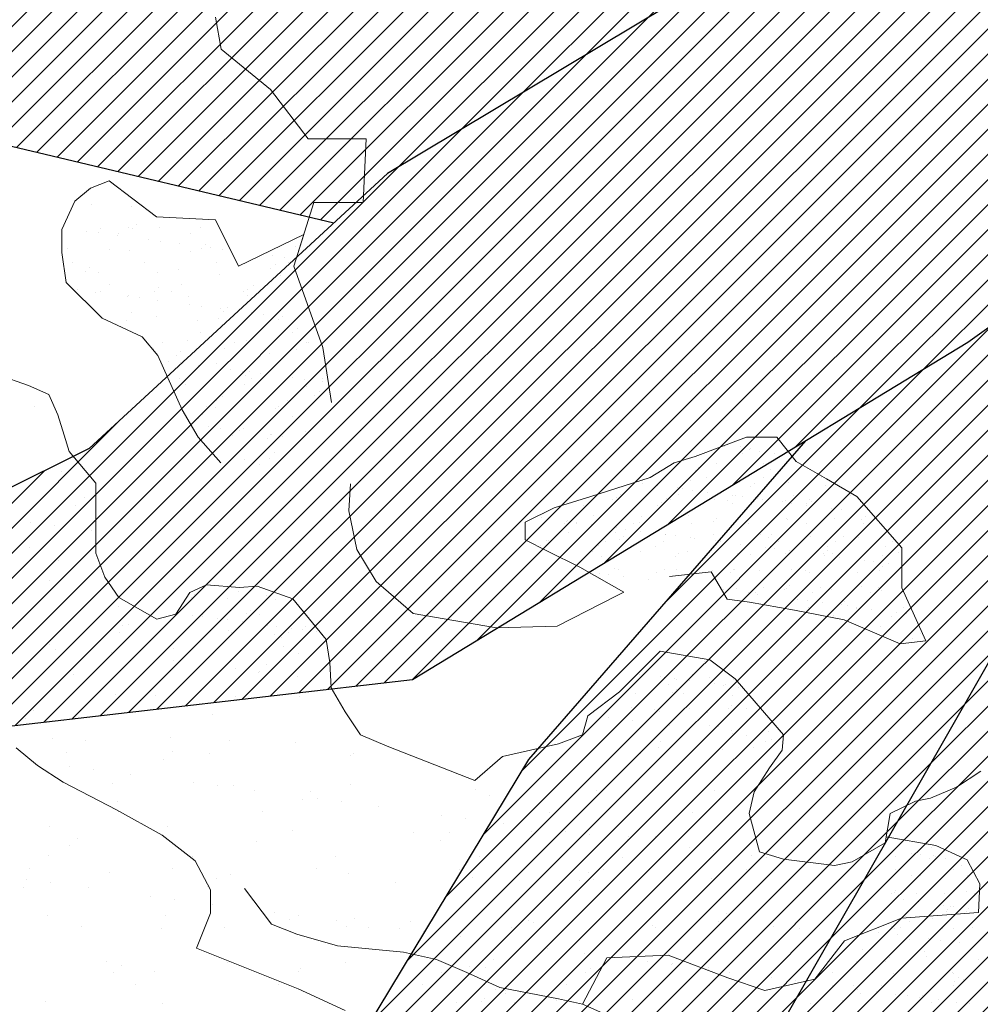
# Model space of a CAD drawing. Units: inches. Extents: x 1986 to 21484, y -1816 to 2016.
# Tile 15 of 85: x 2158.236 to 2166.564, y 1873.899 to 1882.437. Entities that reach past the tile are written whole.
import ezdxf

# ---------------------------------------------------------------- set-up
doc = ezdxf.new("R2010")
doc.units = ezdxf.units.IN
doc.layers.add('L-PLNT', color=84, linetype='Continuous', lineweight=13)
doc.layers.add('vfolhas', color=114, linetype='Continuous', lineweight=5)
for name, color, linetype in [('vfolha', 72, 'Continuous'), ('vfolha2', 110, 'Continuous'), ('vfolhas2', 102, 'Continuous')]:
    doc.layers.add(name, color=color, linetype=linetype)
pattern_1 = [(45, (-2446.5133113, 50.986076), (-0.004419417382, 0.004419417382), [])]

# ---------------------------------------------------------------- blocks, each defined once
blk = doc.blocks.new('arbusto_PB_verde_grande')
at = {"layer": 'vfolha2'}
h = blk.add_hatch(dxfattribs=at)
h.set_pattern_fill('ANSI31', color=256, scale=0.05, style=0)
h.set_pattern_definition(pattern_1)
h.paths.add_polyline_path([(0.02944, 0.35651), (0.00028, 0.09048), (0.02625, -0.03934), (0.047, 0.06233), (0.06189, 0.09731), (0.09372, 0.26573), (0.09955, 0.43473), (0.08789, 0.61313), (0.0645, 0.72266), (0.04988, 0.6851), (0.0236, 0.51294)])
h.paths.add_polyline_path([(0.30106, 0.43789), (0.14225, 0.24871), (0.26685, 0.30022)])
h.paths.add_polyline_path([(0.37995, 0.22817), (0.23697, 0.15193), (0.18428, 0.09364), (0.11122, 0.04358), (0.02625, -0.03934), (0.28061, 0.04667), (0.36829, 0.07798), (0.46756, 0.11239), (0.61068, 0.19376), (0.71585, 0.27823), (0.55813, 0.25948)])
h.paths.add_polyline_path([(0.56101, -0.29441), (0.72752, -0.32573), (0.59024, -0.2412), (0.42962, -0.15982), (0.02625, -0.03934), (0.14922, -0.14107), (0.18838, -0.16604), (0.41501, -0.24435)])
h.paths.add_polyline_path([(-0.27429, -0.44776), (-0.30352, -0.72628), (-0.23923, -0.64175), (-0.15457, -0.45716), (0.02625, -0.03934), (-0.16328, -0.25376)])
h.paths.add_polyline_path([(-0.51963, -0.24744), (-0.67736, -0.32573), (-0.59558, -0.35072), (-0.40574, -0.32882), (-0.21007, -0.20995), (0.02625, -0.03934), (-0.14874, -0.06595), (-0.31518, -0.09101), (-0.41452, -0.15048)])
h.paths.add_polyline_path([(-0.52546, 0.25007), (-0.70947, 0.24698), (-0.51963, 0.1093), (-0.32979, 0.02167), (-0.07567, -0.0128), (-0.04234, -0.02148), (-0.35024, 0.1312)])
at = {"layer": 'vfolhas'}
h = blk.add_hatch(dxfattribs=at)
h.set_pattern_fill('ANSI31', color=256, scale=0.05, style=0)
h.set_pattern_definition(pattern_1)
h.paths.add_polyline_path([(-0.57219, 0.06233), (-0.7153, 0.10298), (-0.67736, 0.08107), (-0.62769, 0.01536), (-0.56347, -0.04095), (-0.26461, -0.0834), (-0.14874, -0.06595), (-0.10151, -0.05877), (-0.20418, -0.0472), (-0.40279, -0.00339)])
h.paths.add_polyline_path([(-0.56347, -0.04095), (-0.58279, -0.02401), (-0.72992, -0.09726), (-0.4334, -0.1679), (-0.41452, -0.15048), (-0.31518, -0.09101), (-0.26461, -0.0834)])
h.paths.add_polyline_path([(-0.2769, -0.47267), (-0.27429, -0.44776), (-0.16328, -0.25376), (0.02625, -0.03934), (-0.21007, -0.20995), (-0.2672, -0.24466), (-0.36485, -0.35697), (-0.42907, -0.46341), (-0.47586, -0.60425), (-0.37946, -0.57603)])
at = {"layer": 'vfolha'}
blk.add_line((-0.2672, -0.24466), (-0.36485, -0.35697), dxfattribs=at)
at = {"layer": 'vfolha2'}
for p, q in [((-0.21007, -0.20995), (0.02625, -0.03934)), ((-0.31518, -0.09101), (-0.41452, -0.15048)), ((-0.41452, -0.15048), (-0.51963, -0.24744)), ((-0.40574, -0.32882), (-0.21007, -0.20995)), ((-0.51963, -0.24744), (-0.67736, -0.32573)), ((-0.16328, -0.25376), (-0.27429, -0.44776)), ((-0.59558, -0.35072), (-0.40574, -0.32882))]:
    blk.add_line(p, q, dxfattribs=at)
at = {"layer": 'vfolhas2'}
for p, q in [((-0.72992, -0.09726), (-0.4334, -0.1679)), ((-0.36485, -0.35697), (-0.42907, -0.46341))]:
    blk.add_line(p, q, dxfattribs=at)
blk = doc.blocks.new('PLANT-SHRUB')
for p, q in [((2159.933, 1882.4585), (2159.9833, 1882.1822)), ((2159.9833, 1882.1822), (2160.4105, 1881.8306)), ((2159.9833, 1882.1822), (2159.9833, 1882.1822)), ((2160.4105, 1881.8306), (2160.7373, 1881.4037)), ((2160.4105, 1881.8306), (2160.4105, 1881.8306)), ((2160.7373, 1881.4037), (2161.24, 1881.4037)), ((2161.24, 1881.4037), (2161.2149, 1880.8511)), ((2159.0126, 1881.0382), (2158.8512, 1880.9762)), ((2159.4223, 1880.7281), (2159.0126, 1881.0382)), ((2158.8512, 1880.9762), (2158.7146, 1880.8646)), ((2158.7146, 1880.8646), (2158.6029, 1880.6164)), ((2160.7876, 1880.8511), (2160.6116, 1880.2986)), ((2161.2149, 1880.8511), (2160.7876, 1880.8511)), ((2158.8595, 1880.8325), (2158.8595, 1880.8325)), ((2159.2032, 1880.8173), (2159.2032, 1880.8173)), ((2159.933, 1880.7004), (2159.4223, 1880.7281)), ((2159.933, 1880.7004), (2159.933, 1880.7004)), ((2160.1341, 1880.2986), (2159.933, 1880.7004)), ((2158.6029, 1880.6164), (2158.6029, 1880.4179)), ((2158.8149, 1880.6018), (2158.8149, 1880.6018)), ((2158.9189, 1880.5881), (2158.9189, 1880.5881)), ((2158.9329, 1880.6299), (2158.9329, 1880.6299)), ((2159.0941, 1880.5844), (2159.0941, 1880.5844)), ((2159.1784, 1880.6381), (2159.1784, 1880.6381)), ((2159.2123, 1880.6297), (2159.2123, 1880.6297)), ((2159.2491, 1880.6634), (2159.2491, 1880.6634)), ((2159.4441, 1880.6323), (2159.4441, 1880.6323)), ((2159.7165, 1880.5832), (2159.7165, 1880.5832)), ((2159.8007, 1880.6369), (2159.8007, 1880.6369)), ((2159.0813, 1880.5667), (2159.0813, 1880.5667)), ((2159.3528, 1880.5309), (2159.3528, 1880.5309)), ((2159.4568, 1880.5173), (2159.4568, 1880.5173)), ((2160.6996, 1880.5749), (2160.1341, 1880.2986)), ((2160.6116, 1880.2986), (2160.6996, 1880.5749)), ((2160.6996, 1880.5749), (2160.6996, 1880.5749)), ((2158.6029, 1880.4179), (2158.6401, 1880.1574)), ((2158.6508, 1880.4516), (2158.6508, 1880.4516)), ((2159.0134, 1880.4474), (2159.0134, 1880.4474)), ((2159.1906, 1880.4322), (2159.1906, 1880.4322)), ((2159.6193, 1880.4959), (2159.6193, 1880.4959)), ((2159.7137, 1880.4255), (2159.7137, 1880.4255)), ((2159.813, 1880.4543), (2159.813, 1880.4543)), ((2159.8498, 1880.488), (2159.8498, 1880.488)), ((2159.8907, 1880.4601), (2159.8907, 1880.4601)), ((2159.9947, 1880.4464), (2159.9947, 1880.4464)), ((2160.6244, 1880.472), (2160.6244, 1880.472)), ((2158.6981, 1880.3321), (2158.6981, 1880.3321)), ((2159.3204, 1880.3309), (2159.3204, 1880.3309)), ((2159.9427, 1880.3298), (2159.9427, 1880.3298)), ((2160.4286, 1880.3893), (2160.4286, 1880.3893)), ((2160.5326, 1880.3756), (2160.5326, 1880.3756)), ((2160.565, 1880.3287), (2160.565, 1880.3287)), ((2158.8027, 1880.2544), (2158.8027, 1880.2544)), ((2158.8395, 1880.2881), (2158.8395, 1880.2881)), ((2158.9203, 1880.2448), (2158.9203, 1880.2448)), ((2159.4315, 1880.2473), (2159.4315, 1880.2473)), ((2159.6141, 1880.272), (2159.6141, 1880.272)), ((2160.1341, 1880.2986), (2160.1341, 1880.2986)), ((2160.4137, 1880.2789), (2160.4137, 1880.2789)), ((2160.4506, 1880.3126), (2160.4506, 1880.3126)), ((2160.6116, 1880.2986), (2160.863, 1879.5954)), ((2160.6116, 1880.2986), (2160.6116, 1880.2986)), ((2158.6401, 1880.1574), (2158.9505, 1879.8472)), ((2159.9713, 1880.2278), (2159.9713, 1880.2278)), ((2160.4944, 1880.2212), (2160.4944, 1880.2212)), ((2158.7346, 1880.0949), (2158.7346, 1880.0949)), ((2158.8971, 1880.0735), (2158.8971, 1880.0735)), ((2158.9328, 1880.084), (2158.9328, 1880.084)), ((2159.017, 1880.1377), (2159.017, 1880.1377)), ((2159.4034, 1880.079), (2159.4034, 1880.079)), ((2159.4402, 1880.1127), (2159.4402, 1880.1127)), ((2159.5551, 1880.0828), (2159.5551, 1880.0828)), ((2159.6393, 1880.1365), (2159.6393, 1880.1365)), ((2160.1774, 1880.0817), (2160.1774, 1880.0817)), ((2160.2148, 1880.0966), (2160.2148, 1880.0966)), ((2160.2617, 1880.1354), (2160.2617, 1880.1354)), ((2159.1685, 1880.0378), (2159.1685, 1880.0378)), ((2159.178, 1880.0472), (2159.178, 1880.0472)), ((2159.2725, 1880.0241), (2159.2725, 1880.0241)), ((2159.435, 1880.0027), (2159.435, 1880.0027)), ((2159.7011, 1880.0405), (2159.7011, 1880.0405)), ((2160.2123, 1880.0429), (2160.2123, 1880.0429)), ((2159.7064, 1879.967), (2159.7064, 1879.967)), ((2159.8105, 1879.9533), (2159.8105, 1879.9533)), ((2159.9729, 1879.9319), (2159.9729, 1879.9319)), ((2160.0041, 1879.9036), (2160.0041, 1879.9036)), ((2160.041, 1879.9373), (2160.041, 1879.9373)), ((2158.9505, 1879.8472), (2159.2982, 1879.686)), ((2159.159, 1879.8305), (2159.159, 1879.8305)), ((2159.2045, 1879.8967), (2159.2045, 1879.8967)), ((2159.419, 1879.8622), (2159.419, 1879.8622)), ((2159.7813, 1879.8294), (2159.7813, 1879.8294)), ((2159.9587, 1879.8428), (2159.9587, 1879.8428)), ((2160.2444, 1879.8962), (2160.2444, 1879.8962)), ((2160.3484, 1879.8825), (2160.3484, 1879.8825)), ((2160.4036, 1879.8283), (2160.4036, 1879.8283)), ((2160.4818, 1879.8361), (2160.4818, 1879.8361)), ((2160.5108, 1879.8611), (2160.5108, 1879.8611)), ((2160.6417, 1879.7619), (2160.6417, 1879.7619)), ((2159.2982, 1879.686), (2159.4348, 1879.5247)), ((2159.6885, 1879.6554), (2159.6885, 1879.6554)), ((2159.8052, 1879.7213), (2159.8052, 1879.7213)), ((2160.1997, 1879.6579), (2160.1997, 1879.6579)), ((2160.6049, 1879.7282), (2160.6049, 1879.7282)), ((2159.3937, 1879.5824), (2159.3937, 1879.5824)), ((2159.4779, 1879.6361), (2159.4779, 1879.6361)), ((2159.6314, 1879.562), (2159.6314, 1879.562)), ((2160.016, 1879.5813), (2160.016, 1879.5813)), ((2160.1003, 1879.635), (2160.1003, 1879.635)), ((2160.6383, 1879.5802), (2160.6383, 1879.5802)), ((2160.7226, 1879.6339), (2160.7226, 1879.6339)), ((2160.7394, 1879.6384), (2160.7394, 1879.6384)), ((2160.863, 1879.5954), (2160.9384, 1879.1182)), ((2159.4348, 1879.5247), (2159.6458, 1879.0532)), ((2159.4348, 1879.5247), (2159.4348, 1879.5247)), ((2159.5222, 1879.4738), (2159.5222, 1879.4738)), ((2159.5945, 1879.5283), (2159.5945, 1879.5283)), ((2160.406, 1879.5459), (2160.406, 1879.5459)), ((2159.6262, 1879.4601), (2159.6262, 1879.4601)), ((2159.7887, 1879.4388), (2159.7887, 1879.4388)), ((2159.9461, 1879.4578), (2159.9461, 1879.4578)), ((2160.0601, 1879.403), (2160.0601, 1879.403)), ((2160.1641, 1879.3893), (2160.1641, 1879.3893)), ((2160.4692, 1879.4511), (2160.4692, 1879.4511)), ((2158.0049, 1879.3737), (2158.3132, 1879.2637)), ((2159.6199, 1879.329), (2159.6199, 1879.329)), ((2160.1953, 1879.3529), (2160.1953, 1879.3529)), ((2160.2321, 1879.3866), (2160.2321, 1879.3866)), ((2160.2422, 1879.3278), (2160.2422, 1879.3278)), ((2160.3266, 1879.3679), (2160.3266, 1879.3679)), ((2160.598, 1879.3322), (2160.598, 1879.3322)), ((2160.702, 1879.3185), (2160.702, 1879.3185)), ((2160.8646, 1879.3267), (2160.8646, 1879.3267)), ((2158.3132, 1879.2637), (2158.4894, 1879.1867)), ((2159.6759, 1879.2704), (2159.6759, 1879.2704)), ((2160.1871, 1879.2728), (2160.1871, 1879.2728)), ((2160.7268, 1879.2534), (2160.7268, 1879.2534)), ((2160.8645, 1879.2971), (2160.8645, 1879.2971)), ((2158.4894, 1879.1867), (2158.5664, 1879.0106)), ((2159.9389, 1879.1346), (2159.9389, 1879.1346)), ((2159.9964, 1879.1706), (2159.9964, 1879.1706)), ((2160.5612, 1879.1334), (2160.5612, 1879.1334)), ((2160.796, 1879.1775), (2160.796, 1879.1775)), ((2160.8328, 1879.2112), (2160.8328, 1879.2112)), ((2158.3642, 1879.0832), (2158.3642, 1879.0832)), ((2159.6458, 1879.0532), (2159.7824, 1878.8175)), ((2159.8546, 1879.0809), (2159.8546, 1879.0809)), ((2159.9335, 1879.0727), (2159.9335, 1879.0727)), ((2160.4566, 1879.066), (2160.4566, 1879.066)), ((2160.4769, 1879.0798), (2160.4769, 1879.0798)), ((2158.5664, 1879.0106), (2158.6215, 1878.8346)), ((2159.7857, 1878.9775), (2159.7857, 1878.9775)), ((2159.8225, 1879.0113), (2159.8225, 1879.0113)), ((2160.5971, 1878.9952), (2160.5971, 1878.9952)), ((2159.8759, 1878.9099), (2159.8759, 1878.9099)), ((2159.9799, 1878.8962), (2159.9799, 1878.8962)), ((2160.1745, 1878.8878), (2160.1745, 1878.8878)), ((2158.6215, 1878.8346), (2158.6655, 1878.6916)), ((2159.7824, 1878.8175), (2159.9811, 1878.5942)), ((2160.0809, 1878.8274), (2160.0809, 1878.8274)), ((2160.1423, 1878.8748), (2160.1423, 1878.8748)), ((2160.3864, 1878.8022), (2160.3864, 1878.8022)), ((2160.4138, 1878.8391), (2160.4138, 1878.8391)), ((2160.4233, 1878.8359), (2160.4233, 1878.8359)), ((2160.5178, 1878.8254), (2160.5178, 1878.8254)), ((2160.6803, 1878.804), (2160.6803, 1878.804)), ((2160.7032, 1878.8263), (2160.7032, 1878.8263)), ((2160.7142, 1878.8683), (2160.7142, 1878.8683)), ((2164.0917, 1878.6487), (2164.5363, 1878.8153)), ((2164.5363, 1878.8153), (2164.8003, 1878.8153)), ((2164.8003, 1878.8153), (2164.967, 1878.607)), ((2164.8003, 1878.8153), (2164.8003, 1878.8153)), ((2164.3454, 1878.7354), (2164.3454, 1878.7354)), ((2164.4894, 1878.7345), (2164.4894, 1878.7345)), ((2164.5625, 1878.7068), (2164.5625, 1878.7068)), ((2164.5717, 1878.7149), (2164.5717, 1878.7149)), ((2158.6655, 1878.6916), (2158.8968, 1878.4165)), ((2159.9209, 1878.6877), (2159.9209, 1878.6877)), ((2160.1875, 1878.6199), (2160.1875, 1878.6199)), ((2160.3998, 1878.633), (2160.3998, 1878.633)), ((2160.444, 1878.681), (2160.444, 1878.681)), ((2163.9111, 1878.5931), (2164.0917, 1878.6487)), ((2164.2631, 1878.6802), (2164.2631, 1878.6802)), ((2164.5043, 1878.672), (2164.5043, 1878.672)), ((2164.6457, 1878.6958), (2164.6457, 1878.6958)), ((2164.7757, 1878.6787), (2164.7757, 1878.6787)), ((2164.9028, 1878.6857), (2164.9028, 1878.6857)), ((2159.9811, 1878.5942), (2159.9811, 1878.5942)), ((2160.3155, 1878.5794), (2160.3155, 1878.5794)), ((2163.7026, 1878.4682), (2163.9111, 1878.5931)), ((2164.124, 1878.5527), (2164.124, 1878.5527)), ((2164.2732, 1878.5846), (2164.2732, 1878.5846)), ((2164.6821, 1878.5866), (2164.6821, 1878.5866)), ((2164.7437, 1878.5398), (2164.7437, 1878.5398)), ((2164.967, 1878.607), (2165.231, 1878.4543)), ((2158.5998, 1878.5173), (2158.5998, 1878.5173)), ((2163.1885, 1878.3016), (2163.7026, 1878.4682)), ((2163.7026, 1878.4682), (2163.7026, 1878.4682)), ((2164.0946, 1878.5257), (2164.0946, 1878.5257)), ((2164.1874, 1878.4701), (2164.1874, 1878.4701)), ((2164.6853, 1878.4692), (2164.6853, 1878.4692)), ((2165.1831, 1878.4683), (2165.1831, 1878.4683)), ((2165.231, 1878.4543), (2165.495, 1878.3016)), ((2158.8968, 1878.4165), (2158.8968, 1878.0974)), ((2161.1044, 1878.4126), (2161.0905, 1878.1766)), ((2163.6377, 1878.4146), (2163.6377, 1878.4146)), ((2163.6385, 1878.4401), (2163.6385, 1878.4401)), ((2163.7676, 1878.3975), (2163.7676, 1878.3975)), ((2163.9355, 1878.3799), (2163.9355, 1878.3799)), ((2163.9848, 1878.3689), (2163.9848, 1878.3689)), ((2164.0475, 1878.4421), (2164.0475, 1878.4421)), ((2164.4793, 1878.4265), (2164.4793, 1878.4265)), ((2164.5752, 1878.3854), (2164.5752, 1878.3854)), ((2164.6046, 1878.4124), (2164.6046, 1878.4124)), ((2164.8978, 1878.4212), (2164.8978, 1878.4212)), ((2165.2243, 1878.3995), (2165.2243, 1878.3995)), ((2158.7944, 1878.2944), (2158.7944, 1878.2944)), ((2162.869, 1878.2044), (2163.1885, 1878.3016)), ((2163.1885, 1878.3016), (2163.1885, 1878.3016)), ((2163.4129, 1878.2975), (2163.4129, 1878.2975)), ((2163.4468, 1878.3164), (2163.4468, 1878.3164)), ((2163.8446, 1878.2819), (2163.8446, 1878.2819)), ((2163.9447, 1878.3155), (2163.9447, 1878.3155)), ((2164.068, 1878.358), (2164.068, 1878.358)), ((2164.198, 1878.3409), (2164.198, 1878.3409)), ((2164.4151, 1878.3123), (2164.4151, 1878.3123)), ((2164.4426, 1878.3146), (2164.4426, 1878.3146)), ((2164.4983, 1878.3013), (2164.4983, 1878.3013)), ((2164.6283, 1878.2842), (2164.6283, 1878.2842)), ((2164.6721, 1878.2786), (2164.6721, 1878.2786)), ((2164.9404, 1878.3137), (2164.9404, 1878.3137)), ((2165.4383, 1878.3128), (2165.4383, 1878.3128)), ((2165.495, 1878.3016), (2165.8841, 1877.8573)), ((2158.7207, 1878.2269), (2158.7207, 1878.2269)), ((2162.6189, 1878.0794), (2162.869, 1878.2044)), ((2163.1272, 1878.22), (2163.1272, 1878.22)), ((2163.1272, 1878.22), (2163.1272, 1878.22)), ((2163.3794, 1878.2735), (2163.3794, 1878.2735)), ((2163.7669, 1878.2255), (2163.7669, 1878.2255)), ((2163.7964, 1878.2525), (2163.7964, 1878.2525)), ((2163.8773, 1878.2725), (2163.8773, 1878.2725)), ((2164.2631, 1878.2766), (2164.2631, 1878.2766)), ((2164.3751, 1878.2716), (2164.3751, 1878.2716)), ((2164.416, 1878.2396), (2164.416, 1878.2396)), ((2164.8455, 1878.2556), (2164.8455, 1878.2556)), ((2164.873, 1878.2707), (2164.873, 1878.2707)), ((2164.9287, 1878.2447), (2164.9287, 1878.2447)), ((2165.0558, 1878.2451), (2165.0558, 1878.2451)), ((2165.0586, 1878.2275), (2165.0586, 1878.2275)), ((2165.0852, 1878.2721), (2165.0852, 1878.2721)), ((2165.1039, 1878.263), (2165.1039, 1878.263)), ((2165.2758, 1878.199), (2165.2758, 1878.199)), ((2165.3708, 1878.2698), (2165.3708, 1878.2698)), ((2165.5223, 1878.2577), (2165.5223, 1878.2577)), ((2161.0905, 1878.1766), (2161.1599, 1877.8434)), ((2162.7596, 1878.1163), (2162.7596, 1878.1163)), ((2162.7782, 1878.153), (2162.7782, 1878.153)), ((2163.21, 1878.1374), (2163.21, 1878.1374)), ((2163.6285, 1878.1321), (2163.6285, 1878.1321)), ((2164.0374, 1878.134), (2164.0374, 1878.134)), ((2164.277, 1878.1121), (2164.277, 1878.1121)), ((2164.4692, 1878.1185), (2164.4692, 1878.1185)), ((2164.8877, 1878.1131), (2164.8877, 1878.1131)), ((2165.2966, 1878.1151), (2165.2966, 1878.1151)), ((2165.359, 1878.188), (2165.359, 1878.188)), ((2165.489, 1878.1709), (2165.489, 1878.1709)), ((2165.5658, 1878.1318), (2165.5658, 1878.1318)), ((2158.3275, 1878.0789), (2158.3275, 1878.0789)), ((2158.5356, 1878.0515), (2158.5356, 1878.0515)), ((2158.8968, 1878.0974), (2158.8968, 1877.8113)), ((2162.6189, 1877.9267), (2162.6189, 1878.0794)), ((2162.9587, 1878.0655), (2162.9587, 1878.0655)), ((2162.9587, 1878.0655), (2162.9587, 1878.0655)), ((2162.9767, 1878.0877), (2162.9767, 1878.0877)), ((2162.9767, 1878.0877), (2162.9767, 1878.0877)), ((2162.9881, 1878.0925), (2162.9881, 1878.0925)), ((2162.9881, 1878.0925), (2162.9881, 1878.0925)), ((2163.0599, 1878.0768), (2163.0599, 1878.0768)), ((2163.0599, 1878.0768), (2163.0599, 1878.0768)), ((2163.0626, 1878.0716), (2163.0626, 1878.0716)), ((2163.0626, 1878.0716), (2163.0626, 1878.0716)), ((2163.1899, 1878.0596), (2163.1899, 1878.0596)), ((2163.4071, 1878.0311), (2163.4071, 1878.0311)), ((2163.5604, 1878.0707), (2163.5604, 1878.0707)), ((2163.6078, 1878.0796), (2163.6078, 1878.0796)), ((2164.0583, 1878.0698), (2164.0583, 1878.0698)), ((2164.2475, 1878.0851), (2164.2475, 1878.0851)), ((2164.5561, 1878.0689), (2164.5561, 1878.0689)), ((2164.8966, 1878.0993), (2164.8966, 1878.0993)), ((2165.054, 1878.068), (2165.054, 1878.068)), ((2165.5363, 1878.1048), (2165.5363, 1878.1048)), ((2165.5518, 1878.0671), (2165.5518, 1878.0671)), ((2158.8605, 1878.0087), (2158.8605, 1878.0087)), ((2162.9938, 1877.9875), (2162.9938, 1877.9875)), ((2162.9938, 1877.9875), (2162.9938, 1877.9875)), ((2163.4028, 1877.9895), (2163.4028, 1877.9895)), ((2163.4687, 1877.9522), (2163.4687, 1877.9522)), ((2163.4903, 1878.0201), (2163.4903, 1878.0201)), ((2163.6202, 1878.003), (2163.6202, 1878.003)), ((2163.8346, 1877.9739), (2163.8346, 1877.9739)), ((2163.8374, 1877.9744), (2163.8374, 1877.9744)), ((2163.9206, 1877.9634), (2163.9206, 1877.9634)), ((2164.0506, 1877.9463), (2164.0506, 1877.9463)), ((2164.0884, 1877.9393), (2164.0884, 1877.9393)), ((2164.253, 1877.9686), (2164.253, 1877.9686)), ((2164.662, 1877.9705), (2164.662, 1877.9705)), ((2164.7281, 1877.9448), (2164.7281, 1877.9448)), ((2164.7575, 1877.9718), (2164.7575, 1877.9718)), ((2165.0938, 1877.955), (2165.0938, 1877.955)), ((2165.3772, 1877.959), (2165.3772, 1877.959)), ((2165.5123, 1877.9496), (2165.5123, 1877.9496)), ((2158.3229, 1877.8624), (2158.3229, 1877.8624)), ((2162.8134, 1877.8295), (2162.6189, 1877.9267)), ((2162.7525, 1877.874), (2162.7525, 1877.874)), ((2162.7525, 1877.874), (2162.7525, 1877.874)), ((2162.7995, 1877.9197), (2162.7995, 1877.9197)), ((2162.7995, 1877.9197), (2162.7995, 1877.9197)), ((2162.8199, 1877.917), (2162.8199, 1877.917)), ((2162.8199, 1877.917), (2162.8199, 1877.917)), ((2163.2503, 1877.8731), (2163.2503, 1877.8731)), ((2163.3177, 1877.9161), (2163.3177, 1877.9161)), ((2163.4392, 1877.9252), (2163.4392, 1877.9252)), ((2163.7482, 1877.8722), (2163.7482, 1877.8722)), ((2163.8156, 1877.9152), (2163.8156, 1877.9152)), ((2164.246, 1877.8713), (2164.246, 1877.8713)), ((2164.2677, 1877.9177), (2164.2677, 1877.9177)), ((2164.3134, 1877.9143), (2164.3134, 1877.9143)), ((2164.3509, 1877.9068), (2164.3509, 1877.9068)), ((2164.4809, 1877.8897), (2164.4809, 1877.8897)), ((2164.6981, 1877.8611), (2164.6981, 1877.8611)), ((2164.7439, 1877.8704), (2164.7439, 1877.8704)), ((2164.8113, 1877.9134), (2164.8113, 1877.9134)), ((2165.2417, 1877.8695), (2165.2417, 1877.8695)), ((2165.3091, 1877.9125), (2165.3091, 1877.9125)), ((2165.7396, 1877.8686), (2165.7396, 1877.8686)), ((2165.807, 1877.9116), (2165.807, 1877.9116)), ((2165.8841, 1877.8573), (2165.8841, 1877.5102)), ((2158.8968, 1877.8113), (2158.9739, 1877.6023)), ((2161.1599, 1877.8434), (2161.3267, 1877.5657)), ((2163.0913, 1877.6907), (2162.8134, 1877.8295)), ((2163.1999, 1877.8294), (2163.1999, 1877.8294)), ((2163.2801, 1877.7794), (2163.2801, 1877.7794)), ((2163.6184, 1877.824), (2163.6184, 1877.824)), ((2163.9198, 1877.7849), (2163.9198, 1877.7849)), ((2163.9493, 1877.8119), (2163.9493, 1877.8119)), ((2164.0274, 1877.826), (2164.0274, 1877.826)), ((2164.4591, 1877.8104), (2164.4591, 1877.8104)), ((2164.569, 1877.799), (2164.569, 1877.799)), ((2164.7813, 1877.8501), (2164.7813, 1877.8501)), ((2164.8776, 1877.8051), (2164.8776, 1877.8051)), ((2164.9112, 1877.833), (2164.9112, 1877.833)), ((2165.1284, 1877.8044), (2165.1284, 1877.8044)), ((2165.2087, 1877.8045), (2165.2087, 1877.8045)), ((2165.2116, 1877.7935), (2165.2116, 1877.7935)), ((2165.2381, 1877.8315), (2165.2381, 1877.8315)), ((2165.2866, 1877.807), (2165.2866, 1877.807)), ((2165.3416, 1877.7764), (2165.3416, 1877.7764)), ((2165.7184, 1877.7915), (2165.7184, 1877.7915)), ((2165.8578, 1877.8187), (2165.8578, 1877.8187)), ((2158.5746, 1877.7472), (2158.5746, 1877.7472)), ((2163.4729, 1877.4726), (2163.0913, 1877.6907)), ((2163.3927, 1877.6814), (2163.3927, 1877.6814)), ((2165.5587, 1877.7478), (2165.5587, 1877.7478)), ((2165.6419, 1877.7368), (2165.6419, 1877.7368)), ((2165.7187, 1877.6912), (2165.7187, 1877.6912)), ((2165.7719, 1877.7197), (2165.7719, 1877.7197)), ((2158.9739, 1877.6023), (2159.095, 1877.4262)), ((2163.2597, 1877.6365), (2163.2597, 1877.6365)), ((2163.3429, 1877.6256), (2163.3429, 1877.6256)), ((2163.4313, 1877.6704), (2163.4313, 1877.6704)), ((2163.4729, 1877.6085), (2163.4729, 1877.6085)), ((2163.7607, 1877.6391), (2163.7607, 1877.6391)), ((2163.8245, 1877.6659), (2163.8245, 1877.6659)), ((2164.2306, 1877.649), (2163.8694, 1877.6074)), ((2163.9292, 1877.6695), (2163.9292, 1877.6695)), ((2164.3696, 1877.413), (2164.2306, 1877.649)), ((2164.243, 1877.6605), (2164.243, 1877.6605)), ((2164.4004, 1877.6446), (2164.4004, 1877.6446)), ((2164.427, 1877.6686), (2164.427, 1877.6686)), ((2164.4299, 1877.6716), (2164.4299, 1877.6716)), ((2164.6519, 1877.6625), (2164.6519, 1877.6625)), ((2164.9249, 1877.6676), (2164.9249, 1877.6676)), ((2165.0495, 1877.6587), (2165.0495, 1877.6587)), ((2165.0837, 1877.6469), (2165.0837, 1877.6469)), ((2165.4227, 1877.6667), (2165.4227, 1877.6667)), ((2165.5022, 1877.6416), (2165.5022, 1877.6416)), ((2165.6892, 1877.6642), (2165.6892, 1877.6642)), ((2158.4939, 1877.5754), (2158.4939, 1877.5754)), ((2159.7116, 1877.4703), (2159.8548, 1877.5363)), ((2159.8548, 1877.5363), (2160.1411, 1877.5143)), ((2160.1411, 1877.5143), (2160.2952, 1877.5253)), ((2160.1411, 1877.5143), (2160.1411, 1877.5143)), ((2160.2952, 1877.5253), (2160.6035, 1877.4152)), ((2161.3267, 1877.5657), (2161.6462, 1877.2881)), ((2163.69, 1877.5799), (2163.69, 1877.5799)), ((2164.6822, 1877.513), (2164.6822, 1877.513)), ((2164.9105, 1877.5313), (2164.9105, 1877.5313)), ((2165.18, 1877.5121), (2165.18, 1877.5121)), ((2165.5301, 1877.5184), (2165.5301, 1877.5184)), ((2165.6779, 1877.5112), (2165.6779, 1877.5112)), ((2165.8841, 1877.5102), (2166.0925, 1877.052)), ((2159.095, 1877.4262), (2159.4253, 1877.2392)), ((2159.5905, 1877.2832), (2159.7116, 1877.4703)), ((2159.7256, 1877.4257), (2159.7256, 1877.4257)), ((2159.7551, 1877.4527), (2159.7551, 1877.4527)), ((2160.1341, 1877.4782), (2160.1341, 1877.4782)), ((2160.3748, 1877.4399), (2160.3748, 1877.4399)), ((2162.8967, 1877.177), (2163.4108, 1877.4408)), ((2163.4108, 1877.4408), (2163.4729, 1877.4726)), ((2163.4108, 1877.4408), (2163.4108, 1877.4408)), ((2164.3335, 1877.4952), (2164.3335, 1877.4952)), ((2164.4491, 1877.5024), (2164.4491, 1877.5024)), ((2164.5507, 1877.4666), (2164.5507, 1877.4666)), ((2164.6148, 1877.4701), (2164.6148, 1877.4701)), ((2164.6339, 1877.4556), (2164.6339, 1877.4556)), ((2164.7638, 1877.4385), (2164.7638, 1877.4385)), ((2164.8675, 1877.497), (2164.8675, 1877.497)), ((2164.881, 1877.5043), (2164.881, 1877.5043)), ((2165.1126, 1877.4692), (2165.1126, 1877.4692)), ((2165.2765, 1877.499), (2165.2765, 1877.499)), ((2165.6105, 1877.4683), (2165.6105, 1877.4683)), ((2165.7083, 1877.4835), (2165.7083, 1877.4835)), ((2159.0899, 1877.3518), (2159.0899, 1877.3518)), ((2160.0368, 1877.4146), (2160.0368, 1877.4146)), ((2160.4553, 1877.4093), (2160.4553, 1877.4093)), ((2160.6035, 1877.4152), (2160.8925, 1877.0609)), ((2164.5641, 1877.3852), (2164.3696, 1877.413)), ((2164.5641, 1877.3852), (2164.5641, 1877.3852)), ((2164.9531, 1877.3158), (2164.5641, 1877.3852)), ((2164.7219, 1877.3585), (2164.7219, 1877.3585)), ((2164.981, 1877.4099), (2164.981, 1877.4099)), ((2165.0642, 1877.399), (2165.0642, 1877.399)), ((2165.0736, 1877.3389), (2165.0736, 1877.3389)), ((2165.1942, 1877.3819), (2165.1942, 1877.3819)), ((2165.3616, 1877.3639), (2165.3616, 1877.3639)), ((2165.391, 1877.391), (2165.391, 1877.391)), ((2165.4113, 1877.3533), (2165.4113, 1877.3533)), ((2165.4945, 1877.3423), (2165.4945, 1877.3423)), ((2159.4253, 1877.2392), (2159.5905, 1877.2832)), ((2159.6054, 1877.2898), (2159.6054, 1877.2898)), ((2159.7354, 1877.2727), (2159.7354, 1877.2727)), ((2159.8172, 1877.2764), (2159.8172, 1877.2764)), ((2159.8206, 1877.2647), (2159.8206, 1877.2647)), ((2160.2062, 1877.2854), (2160.2062, 1877.2854)), ((2160.2296, 1877.2667), (2160.2296, 1877.2667)), ((2160.2357, 1877.3124), (2160.2357, 1877.3124)), ((2160.3151, 1877.2755), (2160.3151, 1877.2755)), ((2161.6462, 1877.2881), (2162.3688, 1877.1631)), ((2165.3839, 1877.2325), (2164.9531, 1877.3158)), ((2165.2936, 1877.2664), (2165.2936, 1877.2664)), ((2165.4921, 1877.3336), (2165.4921, 1877.3336)), ((2165.6245, 1877.3252), (2165.6245, 1877.3252)), ((2165.7915, 1877.2655), (2165.7915, 1877.2655)), ((2165.8416, 1877.2966), (2165.8416, 1877.2966)), ((2165.9011, 1877.3355), (2165.9011, 1877.3355)), ((2165.9249, 1877.2857), (2165.9249, 1877.2857)), ((2159.1318, 1877.1866), (2159.1318, 1877.1866)), ((2159.1767, 1877.193), (2159.1767, 1877.193)), ((2159.4253, 1877.2392), (2159.4253, 1877.2392)), ((2159.9526, 1877.2441), (2159.9526, 1877.2441)), ((2160.0358, 1877.2331), (2160.0358, 1877.2331)), ((2160.1657, 1877.216), (2160.1657, 1877.216)), ((2160.3829, 1877.1874), (2160.3829, 1877.1874)), ((2160.4661, 1877.1765), (2160.4661, 1877.1765)), ((2160.6614, 1877.2511), (2160.6614, 1877.2511)), ((2160.7163, 1877.1721), (2160.7163, 1877.1721)), ((2162.3688, 1877.1631), (2162.8967, 1877.177)), ((2165.8702, 1877.0243), (2165.3839, 1877.2325)), ((2165.6982, 1877.1754), (2165.6982, 1877.1754)), ((2165.8422, 1877.2236), (2165.8422, 1877.2236)), ((2165.8716, 1877.2506), (2165.8716, 1877.2506)), ((2159.103, 1877.1255), (2159.103, 1877.1255)), ((2160.0471, 1877.1396), (2160.0471, 1877.1396)), ((2160.0724, 1877.1208), (2160.0724, 1877.1208)), ((2160.4452, 1877.1013), (2160.4452, 1877.1013)), ((2160.5702, 1877.1199), (2160.5702, 1877.1199)), ((2160.5961, 1877.1594), (2160.5961, 1877.1594)), ((2160.6868, 1877.1451), (2160.6868, 1877.1451)), ((2160.8132, 1877.1308), (2160.8132, 1877.1308)), ((2160.8541, 1877.1032), (2160.8541, 1877.1032)), ((2166.0466, 1877.11), (2166.0466, 1877.11)), ((2158.492, 1877.0224), (2158.492, 1877.0224)), ((2158.9632, 1877.0793), (2158.9632, 1877.0793)), ((2160.5028, 1877.077), (2160.5028, 1877.077)), ((2160.5277, 1876.9993), (2160.5277, 1876.9993)), ((2160.8925, 1877.0609), (2160.9255, 1876.8629)), ((2166.0925, 1877.052), (2165.8702, 1877.0243)), ((2165.891, 1877.0275), (2165.891, 1877.0275)), ((2165.9792, 1877.067), (2165.9792, 1877.067)), ((2158.5494, 1876.9771), (2158.5494, 1876.9771)), ((2159.0349, 1876.951), (2159.0349, 1876.951)), ((2159.2429, 1876.9236), (2159.2429, 1876.9236)), ((2159.5718, 1876.982), (2159.5718, 1876.982)), ((2160.6513, 1876.9431), (2160.6513, 1876.9431)), ((2163.4361, 1876.6098), (2163.7885, 1876.9619)), ((2163.7885, 1876.9619), (2164.2179, 1876.8849)), ((2159.5678, 1876.8808), (2159.5678, 1876.8808)), ((2160.3781, 1876.8422), (2160.3781, 1876.8422)), ((2160.9255, 1876.8629), (2160.9366, 1876.6428)), ((2163.9971, 1876.9019), (2163.9971, 1876.9019)), ((2164.1688, 1876.8679), (2164.1688, 1876.8679)), ((2164.2179, 1876.8849), (2164.4382, 1876.7198)), ((2158.7052, 1876.761), (2158.7052, 1876.761)), ((2160.1107, 1876.8093), (2160.1107, 1876.8093)), ((2160.3045, 1876.7747), (2160.3045, 1876.7747)), ((2160.3187, 1876.782), (2160.3187, 1876.782)), ((2163.6084, 1876.7628), (2163.6084, 1876.7628)), ((2163.7943, 1876.7418), (2163.7943, 1876.7418)), ((2164.0665, 1876.7579), (2164.0665, 1876.7579)), ((2160.6436, 1876.7392), (2160.6436, 1876.7392)), ((2163.8255, 1876.7342), (2163.8255, 1876.7342)), ((2163.8587, 1876.6703), (2163.8587, 1876.6703)), ((2163.9087, 1876.7232), (2163.9087, 1876.7232)), ((2163.9261, 1876.7133), (2163.9261, 1876.7133)), ((2164.0387, 1876.7061), (2164.0387, 1876.7061)), ((2164.2128, 1876.7364), (2164.2128, 1876.7364)), ((2164.2559, 1876.6775), (2164.2559, 1876.6775)), ((2164.3391, 1876.6666), (2164.3391, 1876.6666)), ((2164.3565, 1876.6694), (2164.3565, 1876.6694)), ((2164.424, 1876.7124), (2164.424, 1876.7124)), ((2164.4382, 1876.7198), (2164.8566, 1876.2357)), ((2164.4382, 1876.7198), (2164.4382, 1876.7198)), ((2159.0647, 1876.5817), (2159.0647, 1876.5817)), ((2159.4157, 1876.5723), (2159.4157, 1876.5723)), ((2160.9366, 1876.6428), (2161.0577, 1876.4338)), ((2163.1608, 1876.4008), (2163.4361, 1876.6098)), ((2163.5781, 1876.5919), (2163.5781, 1876.5919)), ((2163.898, 1876.6035), (2163.898, 1876.6035)), ((2163.9274, 1876.6305), (2163.9274, 1876.6305)), ((2163.9871, 1876.5938), (2163.9871, 1876.5938)), ((2164.4189, 1876.5783), (2164.4189, 1876.5783)), ((2164.469, 1876.6495), (2164.469, 1876.6495)), ((2160.1109, 1876.5684), (2160.1109, 1876.5684)), ((2160.6604, 1876.5701), (2160.6604, 1876.5701)), ((2164.408, 1876.4902), (2164.408, 1876.4902)), ((2158.3575, 1876.4423), (2158.3575, 1876.4423)), ((2159.9067, 1876.4102), (2159.9067, 1876.4102)), ((2161.0577, 1876.4338), (2161.1898, 1876.2357)), ((2163.1168, 1876.2357), (2163.1608, 1876.4008)), ((2163.5418, 1876.4685), (2163.5418, 1876.4685)), ((2163.7389, 1876.4577), (2163.7389, 1876.4577)), ((2163.7842, 1876.4337), (2163.7842, 1876.4337)), ((2164.0397, 1876.4676), (2164.0397, 1876.4676)), ((2164.2027, 1876.4284), (2164.2027, 1876.4284)), ((2164.3786, 1876.4632), (2164.3786, 1876.4632)), ((2164.5375, 1876.4667), (2164.5375, 1876.4667)), ((2164.6116, 1876.4303), (2164.6116, 1876.4303)), ((2158.2838, 1876.3748), (2158.2838, 1876.3748)), ((2163.3381, 1876.3844), (2163.3381, 1876.3844)), ((2163.5462, 1876.357), (2163.5462, 1876.357)), ((2163.8711, 1876.3143), (2163.8711, 1876.3143)), ((2164.2194, 1876.3174), (2164.2194, 1876.3174)), ((2161.1898, 1876.2357), (2161.4211, 1876.1367)), ((2162.9076, 1876.1587), (2163.1168, 1876.2357)), ((2164.2948, 1876.3121), (2164.2948, 1876.3121)), ((2164.4088, 1876.2702), (2164.4088, 1876.2702)), ((2164.414, 1876.2428), (2164.414, 1876.2428)), ((2164.7253, 1876.2682), (2164.7253, 1876.2682)), ((2164.8273, 1876.2649), (2164.8273, 1876.2649)), ((2164.8566, 1876.2357), (2164.8456, 1876.1037)), ((2158.5242, 1876.207), (2158.5242, 1876.207)), ((2158.809, 1876.1858), (2158.809, 1876.1858)), ((2159.5466, 1876.2119), (2159.5466, 1876.2119)), ((2160.0536, 1876.1836), (2160.0536, 1876.1836)), ((2160.6261, 1876.173), (2160.6261, 1876.173)), ((2162.4231, 1876.0487), (2162.9076, 1876.1587)), ((2163.7875, 1876.1768), (2163.7875, 1876.1768)), ((2164.5388, 1876.2264), (2164.5388, 1876.2264)), ((2164.622, 1876.2154), (2164.622, 1876.2154)), ((2164.7, 1876.1771), (2164.7, 1876.1771)), ((2164.752, 1876.1983), (2164.752, 1876.1983)), ((2158.3918, 1875.9694), (2158.2046, 1876.1235)), ((2158.6404, 1876.0784), (2158.6404, 1876.0784)), ((2159.559, 1876.0916), (2159.559, 1876.0916)), ((2159.8851, 1876.0762), (2159.8851, 1876.0762)), ((2161.1081, 1876.0594), (2161.1081, 1876.0594)), ((2161.1297, 1876.0739), (2161.1297, 1876.0739)), ((2161.4211, 1876.1367), (2162.1808, 1875.8396)), ((2162.7074, 1876.0731), (2162.7074, 1876.0731)), ((2162.7811, 1876.1406), (2162.7811, 1876.1406)), ((2163.619, 1876.0694), (2163.619, 1876.0694)), ((2163.7742, 1876.1257), (2163.7742, 1876.1257)), ((2164.3302, 1876.1085), (2164.3302, 1876.1085)), ((2164.6016, 1876.1223), (2164.6016, 1876.1223)), ((2164.8456, 1876.1037), (2164.7355, 1875.9497)), ((2159.4853, 1876.0241), (2159.4853, 1876.0241)), ((2162.1808, 1875.8396), (2162.4231, 1876.0487)), ((2158.612, 1875.8264), (2158.3918, 1875.9694)), ((2158.6664, 1875.9647), (2158.6664, 1875.9647)), ((2158.8744, 1875.9373), (2158.8744, 1875.9373)), ((2159.1993, 1875.8945), (2159.1993, 1875.8945)), ((2164.7355, 1875.9497), (2164.6033, 1875.7406)), ((2166.3589, 1875.7824), (2166.5677, 1875.9215)), ((2159.0745, 1875.5843), (2158.612, 1875.8264)), ((2159.0395, 1875.8116), (2159.0395, 1875.8116)), ((2159.7422, 1875.823), (2159.7422, 1875.823)), ((2161.1081, 1875.8032), (2161.1081, 1875.8032)), ((2159.9502, 1875.7957), (2159.9502, 1875.7957)), ((2160.0857, 1875.7983), (2160.0857, 1875.7983)), ((2160.2751, 1875.7529), (2160.2751, 1875.7529)), ((2160.7604, 1875.7408), (2160.7604, 1875.7408)), ((2162.1875, 1875.7643), (2162.1875, 1875.7643)), ((2163.2337, 1875.751), (2163.2337, 1875.751)), ((2163.9088, 1875.7224), (2163.9088, 1875.7224)), ((2163.9825, 1875.7899), (2163.9825, 1875.7899)), ((2164.2561, 1875.7559), (2164.2561, 1875.7559)), ((2164.6033, 1875.7406), (2164.5593, 1875.5536)), ((2166.1327, 1875.6868), (2166.3589, 1875.7824)), ((2159.0875, 1875.6595), (2159.0875, 1875.6595)), ((2160.6867, 1875.6733), (2160.6867, 1875.6733)), ((2160.818, 1875.6814), (2160.818, 1875.6814)), ((2161.026, 1875.654), (2161.026, 1875.654)), ((2162.3096, 1875.7086), (2162.3096, 1875.7086)), ((2165.7839, 1875.5525), (2166.0022, 1875.6607)), ((2166.0022, 1875.6607), (2166.1327, 1875.6868)), ((2159.0745, 1875.5843), (2159.0745, 1875.5843)), ((2159.4709, 1875.3643), (2159.0745, 1875.5843)), ((2159.0929, 1875.5715), (2159.0929, 1875.5715)), ((2160.3376, 1875.5693), (2160.3376, 1875.5693)), ((2161.351, 1875.6112), (2161.351, 1875.6112)), ((2162.8268, 1875.5647), (2162.8268, 1875.5647)), ((2164.0715, 1875.5625), (2164.0715, 1875.5625)), ((2164.5593, 1875.5536), (2164.6497, 1875.2224)), ((2165.7398, 1875.2994), (2165.7839, 1875.5525)), ((2161.8938, 1875.5398), (2161.8938, 1875.5398)), ((2162.1019, 1875.5124), (2162.1019, 1875.5124)), ((2162.4268, 1875.4696), (2162.4268, 1875.4696)), ((2158.4991, 1875.4369), (2158.4991, 1875.4369)), ((2159.5215, 1875.4418), (2159.5215, 1875.4418)), ((2160.6009, 1875.4029), (2160.6009, 1875.4029)), ((2161.6471, 1875.3896), (2161.6471, 1875.3896)), ((2161.9619, 1875.39), (2161.9619, 1875.39)), ((2162.6695, 1875.3945), (2162.6695, 1875.3945)), ((2162.9697, 1875.3981), (2162.9697, 1875.3981)), ((2158.7398, 1875.3409), (2158.7398, 1875.3409)), ((2159.7572, 1875.1442), (2159.4709, 1875.3643)), ((2160.2889, 1875.3088), (2160.2889, 1875.3088)), ((2161.8882, 1875.3225), (2161.8882, 1875.3225)), ((2163.1777, 1875.3708), (2163.1777, 1875.3708)), ((2163.5026, 1875.328), (2163.5026, 1875.328)), ((2163.511, 1875.3578), (2163.511, 1875.3578)), ((2163.749, 1875.3556), (2163.749, 1875.3556)), ((2165.4535, 1875.1344), (2165.7398, 1875.2994)), ((2165.7398, 1875.2994), (2165.7398, 1875.2994)), ((2166.1777, 1875.2758), (2165.7487, 1875.3505)), ((2158.6661, 1875.2734), (2158.6661, 1875.2734)), ((2164.0455, 1875.2565), (2164.0455, 1875.2565)), ((2164.2535, 1875.2291), (2164.2535, 1875.2291)), ((2164.6497, 1875.2224), (2164.8589, 1875.1564)), ((2165.9653, 1875.2107), (2165.9653, 1875.2107)), ((2166.1416, 1875.2621), (2166.1416, 1875.2621)), ((2166.4493, 1875.1525), (2166.1777, 1875.2758)), ((2158.4862, 1875.185), (2158.4862, 1875.185)), ((2159.7308, 1875.1827), (2159.7308, 1875.1827)), ((2159.8894, 1874.8912), (2159.7572, 1875.1442)), ((2160.9755, 1875.1805), (2160.9755, 1875.1805)), ((2162.2201, 1875.1782), (2162.2201, 1875.1782)), ((2163.4647, 1875.1759), (2163.4647, 1875.1759)), ((2164.5784, 1875.1863), (2164.5784, 1875.1863)), ((2164.7094, 1875.1737), (2164.7094, 1875.1737)), ((2164.8589, 1875.1564), (2165.2994, 1875.1014)), ((2164.8589, 1875.1564), (2164.8589, 1875.1564)), ((2165.2994, 1875.1014), (2165.4535, 1875.1344)), ((2165.8306, 1875.1793), (2165.8306, 1875.1793)), ((2166.0485, 1875.1998), (2166.0485, 1875.1998)), ((2166.1261, 1875.1611), (2166.1261, 1875.1611)), ((2166.1556, 1875.1881), (2166.1556, 1875.1881)), ((2166.1785, 1875.1826), (2166.1785, 1875.1826)), ((2166.2624, 1875.1637), (2166.2624, 1875.1637)), ((2166.3956, 1875.1541), (2166.3956, 1875.1541)), ((2166.5603, 1874.9428), (2166.4493, 1875.1525)), ((2158.3177, 1875.0776), (2158.3177, 1875.0776)), ((2159.0143, 1875.0415), (2159.0143, 1875.0415)), ((2159.5623, 1875.0754), (2159.5623, 1875.0754)), ((2160.8069, 1875.0731), (2160.8069, 1875.0731)), ((2162.0516, 1875.0708), (2162.0516, 1875.0708)), ((2163.1633, 1875.0392), (2163.1633, 1875.0392)), ((2163.2962, 1875.0686), (2163.2962, 1875.0686)), ((2164.5408, 1875.0663), (2164.5408, 1875.0663)), ((2165.8315, 1875.0645), (2165.8315, 1875.0645)), ((2165.8989, 1875.1075), (2165.8989, 1875.1075)), ((2166.3293, 1875.0636), (2166.3293, 1875.0636)), ((2166.3968, 1875.1066), (2166.3968, 1875.1066)), ((2158.2979, 1874.9784), (2158.2979, 1874.9784)), ((2158.5059, 1874.951), (2158.5059, 1874.951)), ((2159.9412, 1874.9901), (2159.9412, 1874.9901)), ((2160.0605, 1875.0282), (2160.0605, 1875.0282)), ((2161.0829, 1875.0331), (2161.0829, 1875.0331)), ((2161.4904, 1874.958), (2161.4904, 1874.958)), ((2162.1624, 1874.9942), (2162.1624, 1874.9942)), ((2163.0897, 1874.9717), (2163.0897, 1874.9717)), ((2163.2085, 1874.9809), (2163.2085, 1874.9809)), ((2164.2309, 1874.9858), (2164.2309, 1874.9858)), ((2164.7125, 1875.0071), (2164.7125, 1875.0071)), ((2165.967, 1875.0153), (2165.967, 1875.0153)), ((2166.0462, 1875.0138), (2166.0462, 1875.0138)), ((2166.4552, 1875.0158), (2166.4552, 1875.0158)), ((2158.2683, 1874.9089), (2158.2683, 1874.9089)), ((2158.8308, 1874.9082), (2158.8308, 1874.9082)), ((2159.8676, 1874.9226), (2159.8676, 1874.9226)), ((2159.8896, 1874.6886), (2159.8894, 1874.8912)), ((2160.1867, 1874.9022), (2160.4179, 1874.5941)), ((2165.3104, 1874.9469), (2165.3104, 1874.9469)), ((2165.8205, 1874.8712), (2165.8205, 1874.8712)), ((2165.8279, 1874.8879), (2165.8279, 1874.8879)), ((2166.4476, 1874.875), (2166.4476, 1874.875)), ((2166.548, 1874.6962), (2166.5603, 1874.9428)), ((2159.3737, 1874.8367), (2159.3737, 1874.8367)), ((2159.5817, 1874.8094), (2159.5817, 1874.8094)), ((2165.7985, 1874.8609), (2165.7985, 1874.8609)), ((2165.9011, 1874.8052), (2165.9011, 1874.8052)), ((2166.0125, 1874.8617), (2166.0125, 1874.8617)), ((2166.0311, 1874.7881), (2166.0311, 1874.7881)), ((2166.2523, 1874.8557), (2166.2523, 1874.8557)), ((2166.5103, 1874.8608), (2166.5103, 1874.8608)), ((2159.9066, 1874.7666), (2159.9066, 1874.7666)), ((2160.4495, 1874.6951), (2160.4495, 1874.6951)), ((2165.8816, 1874.6469), (2166.548, 1874.6962)), ((2166.2482, 1874.7595), (2166.2482, 1874.7595)), ((2166.2676, 1874.7062), (2166.2676, 1874.7062)), ((2166.2791, 1874.7205), (2166.2791, 1874.7205)), ((2166.3085, 1874.7475), (2166.3085, 1874.7475)), ((2166.3315, 1874.7486), (2166.3315, 1874.7486)), ((2166.4451, 1874.7077), (2166.4451, 1874.7077)), ((2166.4614, 1874.7315), (2166.4614, 1874.7315)), ((2158.4739, 1874.6668), (2158.4739, 1874.6668)), ((2159.4963, 1874.6717), (2159.4963, 1874.6717)), ((2159.7682, 1874.385), (2159.8896, 1874.6886)), ((2159.8896, 1874.6886), (2159.8896, 1874.6886)), ((2160.5758, 1874.6328), (2160.5758, 1874.6328)), ((2160.6575, 1874.6677), (2160.6575, 1874.6677)), ((2160.9825, 1874.6249), (2160.9825, 1874.6249)), ((2161.1427, 1874.6394), (2161.1427, 1874.6394)), ((2161.6219, 1874.6195), (2161.6219, 1874.6195)), ((2162.6443, 1874.6244), (2162.6443, 1874.6244)), ((2162.6919, 1874.6072), (2162.6919, 1874.6072)), ((2164.2911, 1874.6209), (2164.2911, 1874.6209)), ((2164.3648, 1874.6884), (2164.3648, 1874.6884)), ((2165.3879, 1874.4496), (2165.8816, 1874.6469)), ((2165.914, 1874.6563), (2165.914, 1874.6563)), ((2165.9541, 1874.6173), (2165.9541, 1874.6173)), ((2166.148, 1874.6455), (2166.148, 1874.6455)), ((2158.7702, 1874.5707), (2158.7702, 1874.5707)), ((2159.4698, 1874.5581), (2159.4698, 1874.5581)), ((2160.0148, 1874.5685), (2160.0148, 1874.5685)), ((2160.4179, 1874.5941), (2160.6381, 1874.5061)), ((2161.069, 1874.5719), (2161.069, 1874.5719)), ((2161.2594, 1874.5662), (2161.2594, 1874.5662)), ((2161.5253, 1874.5535), (2161.5253, 1874.5535)), ((2161.7334, 1874.5261), (2161.7334, 1874.5261)), ((2162.5041, 1874.5639), (2162.5041, 1874.5639)), ((2163.7238, 1874.5855), (2163.7238, 1874.5855)), ((2163.7487, 1874.5617), (2163.7487, 1874.5617)), ((2164.77, 1874.5721), (2164.77, 1874.5721)), ((2164.9933, 1874.5594), (2164.9933, 1874.5594)), ((2165.683, 1874.5235), (2165.683, 1874.5235)), ((2165.7924, 1874.577), (2165.7924, 1874.577)), ((2165.8209, 1874.5551), (2165.8209, 1874.5551)), ((2165.8699, 1874.5636), (2165.8699, 1874.5636)), ((2166.238, 1874.5571), (2166.238, 1874.5571)), ((2166.3321, 1874.5576), (2166.3321, 1874.5576)), ((2166.4922, 1874.5625), (2166.4922, 1874.5625)), ((2160.6381, 1874.5061), (2160.9905, 1874.407)), ((2162.0583, 1874.4833), (2162.0583, 1874.4833)), ((2165.1287, 1874.1166), (2165.3879, 1874.4496)), ((2165.8455, 1874.5021), (2165.8455, 1874.5021)), ((2165.9491, 1874.4632), (2165.9491, 1874.4632)), ((2166.1169, 1874.4664), (2166.1169, 1874.4664)), ((2166.2209, 1874.4527), (2166.2209, 1874.4527)), ((2160.6491, 1874.0329), (2159.7682, 1874.385)), ((2160.9905, 1874.407), (2161.5631, 1874.352)), ((2161.5631, 1874.352), (2161.8494, 1874.286)), ((2162.6012, 1874.4118), (2162.6012, 1874.4118)), ((2162.8092, 1874.3845), (2162.8092, 1874.3845)), ((2165.5388, 1874.3769), (2165.5388, 1874.3769)), ((2166.0785, 1874.3575), (2166.0785, 1874.3575)), ((2166.3834, 1874.4313), (2166.3834, 1874.4313)), ((2158.9892, 1874.2714), (2158.9892, 1874.2714)), ((2161.8494, 1874.286), (2162.1136, 1874.176)), ((2162.3442, 1874.2886), (2162.3442, 1874.2886)), ((2163.1157, 1873.9009), (2163.3269, 1874.3016)), ((2163.1341, 1874.3417), (2163.1341, 1874.3417)), ((2163.3269, 1874.3016), (2163.8576, 1874.3262)), ((2163.677, 1874.2702), (2163.677, 1874.2702)), ((2163.8576, 1874.3262), (2164.3759, 1874.1289)), ((2165.4926, 1874.2702), (2165.4926, 1874.2702)), ((2165.5663, 1874.3377), (2165.5663, 1874.3377)), ((2165.7384, 1874.2702), (2165.7384, 1874.2702)), ((2165.7752, 1874.3039), (2165.7752, 1874.3039)), ((2166.0961, 1874.3102), (2166.0961, 1874.3102)), ((2166.5498, 1874.2878), (2166.5498, 1874.2878)), ((2159.1221, 1874.2395), (2159.1221, 1874.2395)), ((2159.4081, 1874.1819), (2159.4081, 1874.1819)), ((2160.0353, 1874.2581), (2160.0353, 1874.2581)), ((2160.6712, 1874.2073), (2160.6712, 1874.2073)), ((2161.0577, 1874.263), (2161.0577, 1874.263)), ((2162.1372, 1874.2241), (2162.1372, 1874.2241)), ((2162.2705, 1874.2211), (2162.2705, 1874.2211)), ((2163.1834, 1874.2108), (2163.1834, 1874.2108)), ((2163.885, 1874.2428), (2163.885, 1874.2428)), ((2163.8933, 1874.2564), (2163.8933, 1874.2564)), ((2164.2058, 1874.2157), (2164.2058, 1874.2157)), ((2164.2099, 1874.2), (2164.2099, 1874.2)), ((2159.0484, 1874.172), (2159.0484, 1874.172)), ((2160.6527, 1874.1797), (2160.6527, 1874.1797)), ((2161.8973, 1874.1774), (2161.8973, 1874.1774)), ((2162.1136, 1874.176), (2162.3999, 1874.0439)), ((2163.142, 1874.1751), (2163.142, 1874.1751)), ((2164.3759, 1874.1289), (2164.6968, 1874.018)), ((2164.3866, 1874.1729), (2164.3866, 1874.1729)), ((2164.6968, 1874.018), (2165.1287, 1874.1166)), ((2164.7528, 1874.1286), (2164.7528, 1874.1286)), ((2164.9608, 1874.1012), (2164.9608, 1874.1012)), ((2165.2852, 1874.1768), (2165.2852, 1874.1768)), ((2165.6312, 1874.1706), (2165.6312, 1874.1706)), ((2165.7927, 1874.1169), (2165.7927, 1874.1169)), ((2165.8083, 1874.1701), (2165.8083, 1874.1701)), ((2166.3195, 1874.1726), (2166.3195, 1874.1726)), ((2166.3314, 1874.1634), (2166.3314, 1874.1634)), ((2166.3391, 1874.0948), (2166.3391, 1874.0948)), ((2166.376, 1874.1285), (2166.376, 1874.1285)), ((2166.4151, 1874.1158), (2166.4151, 1874.1158)), ((2159.2395, 1874.0745), (2159.2395, 1874.0745)), ((2160.4841, 1874.0723), (2160.4841, 1874.0723)), ((2161.0566, 1873.8459), (2160.6491, 1874.0329)), ((2161.7288, 1874.07), (2161.7288, 1874.07)), ((2162.2693, 1874.0674), (2162.2693, 1874.0674)), ((2162.3634, 1874.0292), (2162.3634, 1874.0292)), ((2162.3999, 1874.0439), (2162.9065, 1873.9449)), ((2162.4466, 1874.0183), (2162.4466, 1874.0183)), ((2162.9734, 1874.0678), (2162.9734, 1874.0678)), ((2164.218, 1874.0655), (2164.218, 1874.0655)), ((2165.2858, 1874.0584), (2165.2858, 1874.0584)), ((2165.4627, 1874.0632), (2165.4627, 1874.0632)), ((2165.4987, 1874.0304), (2165.4987, 1874.0304)), ((2165.5395, 1874.0879), (2165.5395, 1874.0879)), ((2165.6612, 1874.009), (2165.6612, 1874.009)), ((2165.7085, 1874.0632), (2165.7085, 1874.0632)), ((2166.3308, 1874.0621), (2166.3308, 1874.0621)), ((2162.2672, 1873.9478), (2162.2672, 1873.9478)), ((2162.4444, 1873.9883), (2162.4444, 1873.9883)), ((2162.5766, 1874.0012), (2162.5766, 1874.0012)), ((2162.8869, 1873.935), (2162.8869, 1873.935)), ((2162.9065, 1873.9449), (2163.1157, 1873.9009)), ((2163.5456, 1873.9378), (2163.5456, 1873.9378)), ((2165.3656, 1873.9286), (2165.3656, 1873.9286)), ((2165.5262, 1873.9919), (2165.5262, 1873.9919)), ((2165.8286, 1873.9869), (2165.8286, 1873.9869)), ((2165.9326, 1873.9732), (2165.9326, 1873.9732)), ((2166.0367, 1873.9596), (2166.0367, 1873.9596)), ((2166.0367, 1873.9596), (2166.0367, 1873.9596)), ((2166.0659, 1873.9724), (2166.0659, 1873.9724)), ((2166.1991, 1873.9382), (2166.1991, 1873.9382)), ((2158.4623, 1873.9219), (2158.4623, 1873.9219)), ((2159.4711, 1873.9016), (2159.4711, 1873.9016)), ((2162.0266, 1873.9128), (2162.0266, 1873.9128)), ((2162.2378, 1873.9208), (2162.2378, 1873.9208)), ((2162.5244, 1873.9119), (2162.5244, 1873.9119)), ((2163.0223, 1873.911), (2163.0223, 1873.911)), ((2163.1157, 1873.9009), (2163.5892, 1873.6919)), ((2165.0948, 1873.9056), (2165.0948, 1873.9056)), ((2166.1402, 1873.9125), (2166.1402, 1873.9125)), ((2166.3616, 1873.9168), (2166.3616, 1873.9168)), ((2166.4706, 1873.9024), (2166.4706, 1873.9024))]:
    blk.add_line(p, q)

msp = doc.modelspace()

# ---------------------------------------------------------------- block references
at = {"layer": 'L-PLNT'}
msp.add_blockref('PLANT-SHRUB', (0, 0), dxfattribs=at)
at = {"layer": 'L-PLNT', "xscale": 24.60366729364114, "yscale": 24.60366729364114, "zscale": 24.60366729364114}
msp.add_blockref('arbusto_PB_verde_grande', (2171.6234, 1884.8051), dxfattribs=at)

doc.saveas('drawing.dxf')
